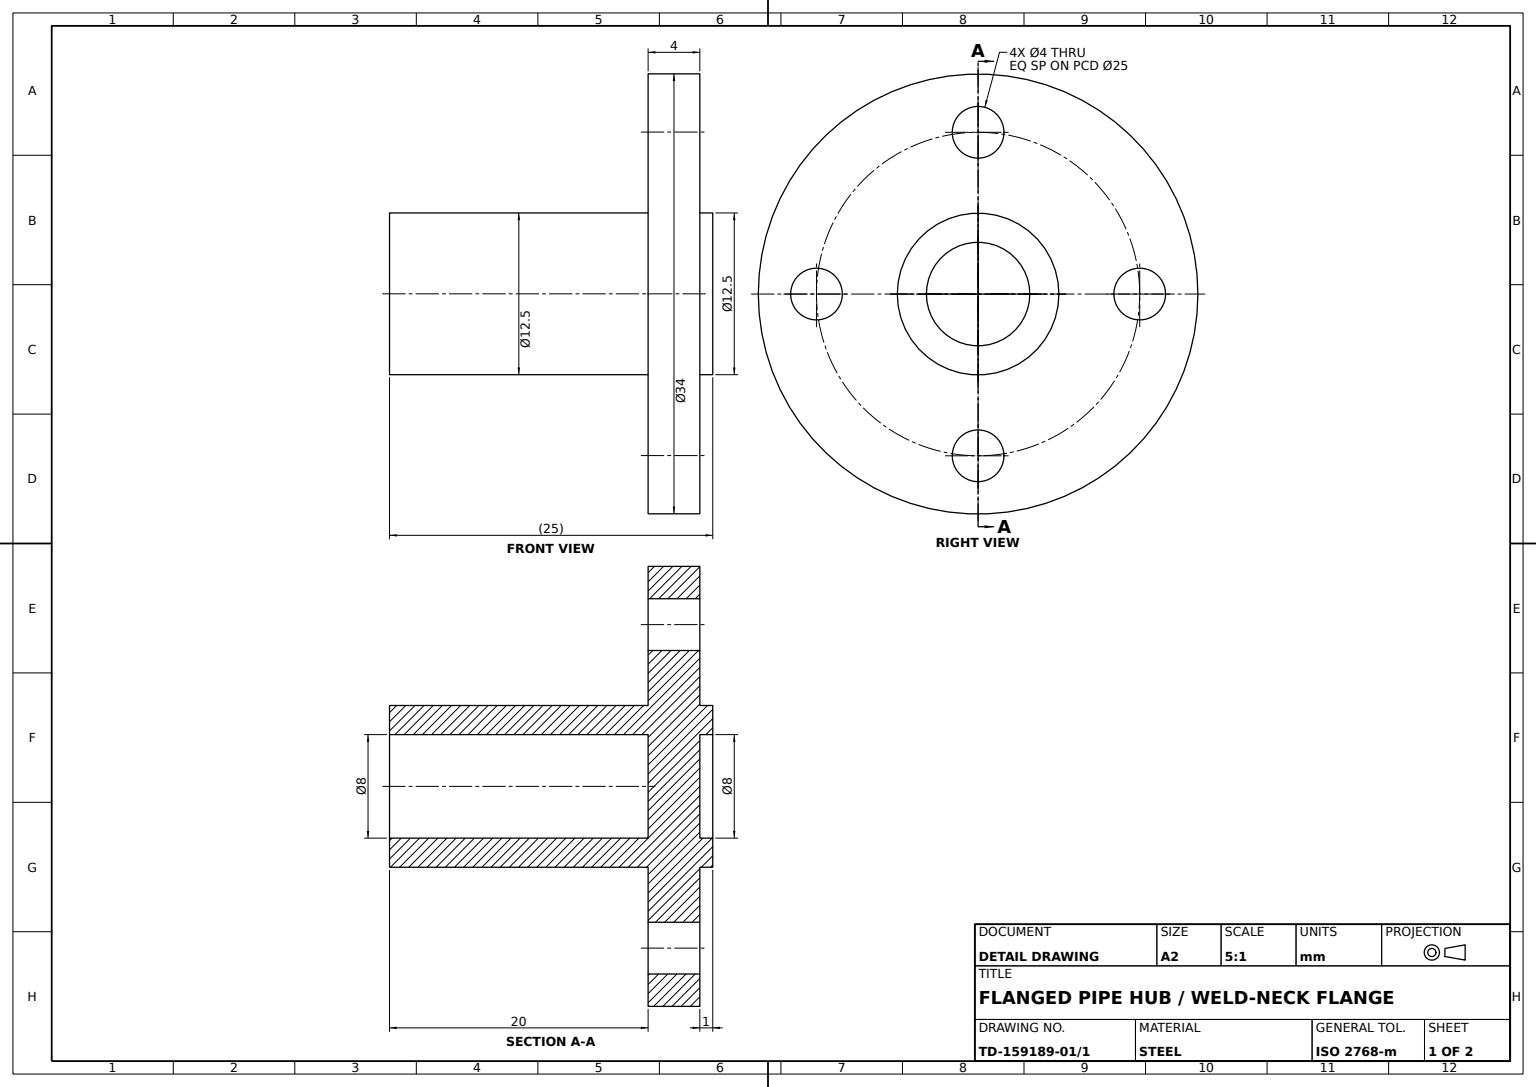
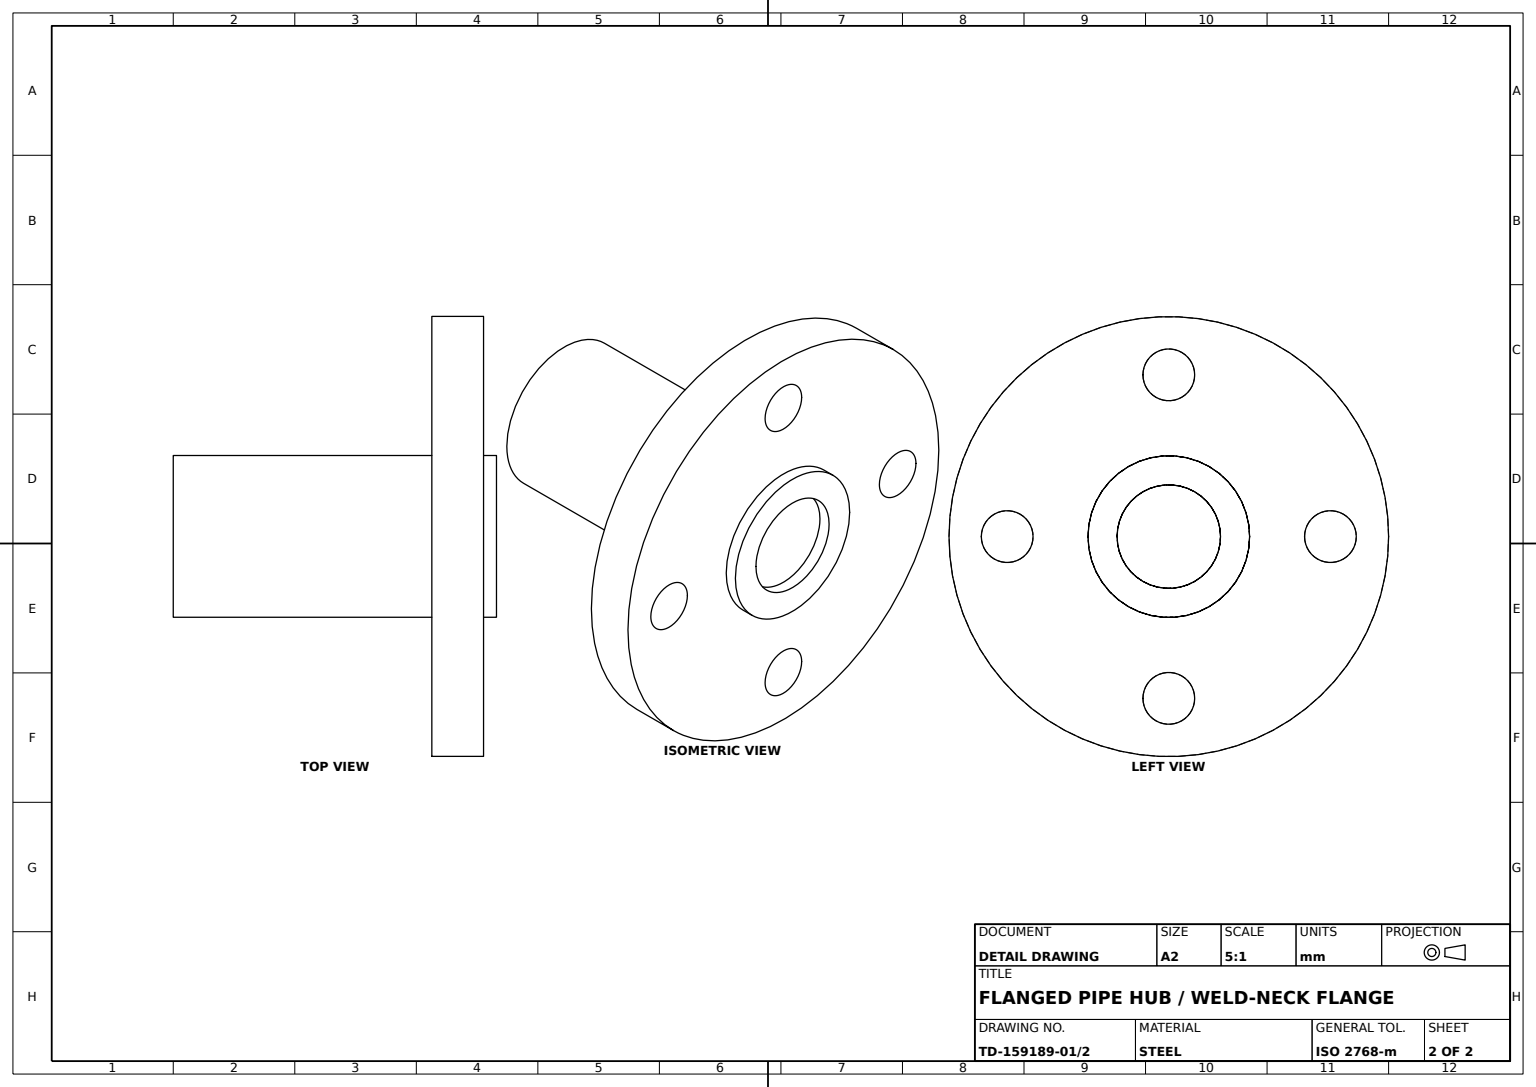
SolidWorks part; units mm, degrees
material "Plain Carbon Steel"
ref_plane "Front Plane" through (0, 0, 0) normal (0, 0, 1) x (1, 0, 0)
ref_plane "Top Plane" through (0, 0, 0) normal (0, 1, 0) x (1, 0, 0)
ref_plane "Right Plane" through (0, 0, 0) normal (1, 0, 0) x (0, 0, -1)
sketch "Flange Profile Sketch" plane through (0, 0, 0) normal (0, 0, 1) x (1, 0, 0)
  circle A0 centre (0, 0) radius 17
  dimension "D1" = 34
  dimension "D2" = 34
extrude "Flange Ø34x4" add sketch "Flange Profile Sketch" along normal blind 4
sketch "Hub Profile Sketch" plane through (0, 0, 4) normal (0, 0, 1) x (1, 0, 0)
  circle A0 centre (0, 0) radius 6.25
  circle A1 centre (0, 0) radius 4
  dimension "D1" = 12.5
  dimension "D2" = 8
  dimension "D3" = 8
  dimension "D4" = 12.5
extrude "Hub Tube 20mm" add sketch "Hub Profile Sketch" along normal blind 20
sketch "Bolt Holes Sketch" plane through (0, 0, 4) normal (0, 0, 1) x (1, 0, 0)
  circle A1 centre (0, 12.5) radius 2
  circle A2 centre (12.5, 0) radius 2
  circle A3 centre (0, -12.5) radius 2
  circle A4 centre (-12.5, 0) radius 2
  dimension "D1" = 4
  dimension "D2" = 4
  dimension "D3" = 4
  dimension "D4" = 4
  dimension "D5" = 4
  dimension "D6" = 12.5
  dimension "D7" = 12.5
  dimension "D8" = 12.5
  dimension "D9" = 12.5
extrude "Bolt Holes 4x" cut sketch "Bolt Holes Sketch" against normal blind 4
sketch "Rear Spigot Sketch" plane through (0, 0, 0) normal (0, 0, -1) x (-1, 0, 0)
  circle A0 centre (0, 0) radius 6.25
  circle A1 centre (0, 0) radius 4
  dimension "D1" = 12.5
  dimension "D2" = 8
  dimension "D3" = 8
  dimension "D4" = 12.5
extrude "Rear Spigot 1mm" add sketch "Rear Spigot Sketch" along normal blind 1
